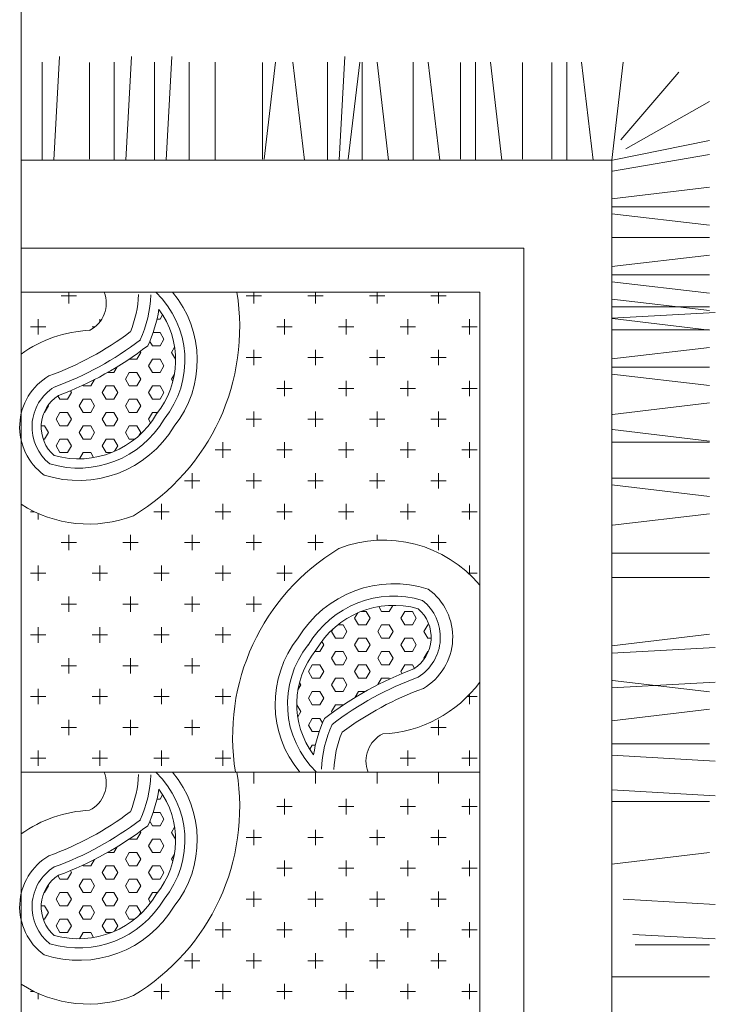
# Model space of a CAD drawing. Units: inches. Extents: x -638 to 186, y -762 to 59.
# Tile 26 of 31: x -65.1 to -52.81, y -94 to -76.62. Entities that reach past the tile are written whole.
import ezdxf

# ---------------------------------------------------------------- set-up
doc = ezdxf.new("R2010")
doc.units = ezdxf.units.IN
doc.layers.add('furn', color=8, linetype='Continuous', lineweight=13)

# ---------------------------------------------------------------- blocks, each defined once
blk = doc.blocks.new('BED-DOUBLE-WITH-NIGHTSTANDS')
for p, q in [((58.548, 11.244), (58.548, 59.951)), ((59.126, 31.914), (59.228, 33.743)), ((60.397, 31.914), (60.499, 33.743)), ((61.11, 31.914), (61.212, 33.743)), ((64.165, 31.914), (64.266, 33.743)), ((58.923, 31.914), (58.923, 33.642)), ((59.755, 31.928), (59.755, 33.639)), ((60.193, 31.914), (60.193, 33.642)), ((60.906, 31.914), (60.906, 33.642)), ((61.517, 31.914), (61.517, 33.642)), ((61.977, 31.914), (61.977, 33.642)), ((62.81, 31.928), (62.81, 33.639)), ((62.841, 31.928), (63.044, 33.642)), ((63.554, 31.914), (63.35, 33.642)), ((63.961, 31.914), (63.961, 33.642)), ((64.327, 31.928), (64.531, 33.642)), ((64.572, 31.914), (64.572, 33.642)), ((65.04, 31.914), (64.836, 33.642)), ((65.476, 31.914), (65.476, 33.642)), ((65.944, 31.914), (65.741, 33.642)), ((66.309, 31.928), (66.309, 33.639)), ((66.573, 31.914), (66.573, 33.642)), ((67.041, 31.914), (66.838, 33.642)), ((67.406, 31.928), (67.406, 33.639)), ((67.922, 31.928), (67.922, 33.639)), ((68.186, 31.914), (68.186, 33.642)), ((68.654, 31.914), (68.45, 33.642)), ((68.982, 31.914), (69.186, 33.642)), ((69.142, 32.273), (70.169, 33.468)), ((69.232, 32.112), (70.71, 32.951)), ((68.996, 31.914), (70.707, 32.257)), ((68.996, 31.721), (70.707, 32.011)), ((58.548, 31.914), (68.982, 31.914)), ((68.982, 31.914), (68.982, 1.829)), ((68.982, 31.232), (70.71, 31.436)), ((68.982, 30.966), (70.71, 30.762)), ((68.996, 31.086), (70.707, 31.086)), ((68.982, 30.547), (70.71, 30.547)), ((58.548, 30.359), (67.427, 30.359)), ((67.427, 30.359), (67.427, 3.384)), ((68.982, 30.033), (70.71, 30.237)), ((68.982, 29.767), (70.71, 29.563)), ((68.996, 29.887), (70.707, 29.887)), ((58.548, 29.582), (66.65, 29.582)), ((59.394, 29.379), (59.394, 29.582)), ((62.659, 29.379), (62.659, 29.582)), ((63.748, 29.379), (63.748, 29.582)), ((64.836, 29.379), (64.836, 29.582)), ((65.924, 29.379), (65.924, 29.582)), ((66.65, 29.582), (66.65, 4.161)), ((59.258, 29.515), (59.53, 29.515)), ((62.523, 29.515), (62.795, 29.515)), ((63.612, 29.515), (63.884, 29.515)), ((64.7, 29.515), (64.972, 29.515)), ((65.788, 29.515), (66.06, 29.515)), ((68.982, 29.46), (70.71, 29.256)), ((68.982, 29.324), (70.71, 29.324)), ((68.982, 29.121), (70.811, 29.223)), ((58.85, 28.835), (58.85, 29.107)), ((59.938, 29.054), (59.938, 29.107)), ((61.003, 29.104), (60.948, 29.104)), ((61.047, 29.18), (61.003, 29.104)), ((63.203, 28.835), (63.203, 29.107)), ((64.292, 28.835), (64.292, 29.107)), ((65.38, 28.835), (65.38, 29.107)), ((66.468, 28.835), (66.468, 29.107)), ((68.996, 29.116), (70.71, 28.912)), ((58.714, 28.971), (58.986, 28.971)), ((59.802, 28.971), (59.857, 28.971)), ((61.003, 28.869), (60.881, 28.869)), ((61.003, 28.869), (61.072, 28.751)), ((63.067, 28.971), (63.339, 28.971)), ((64.156, 28.971), (64.428, 28.971)), ((65.244, 28.971), (65.516, 28.971)), ((66.332, 28.971), (66.605, 28.971)), ((68.982, 28.917), (70.71, 28.917)), ((60.821, 28.713), (60.867, 28.633)), ((61.072, 28.751), (61.003, 28.633)), ((60.663, 28.515), (60.595, 28.397)), ((60.652, 28.534), (60.663, 28.515)), ((61.003, 28.633), (60.867, 28.633)), ((61.261, 28.608), (61.208, 28.515)), ((61.208, 28.515), (61.276, 28.397)), ((62.659, 28.291), (62.659, 28.563)), ((63.748, 28.291), (63.748, 28.563)), ((64.836, 28.291), (64.836, 28.563)), ((65.924, 28.291), (65.924, 28.563)), ((68.982, 28.403), (70.71, 28.606)), ((60.459, 28.399), (60.459, 28.397)), ((60.595, 28.397), (60.459, 28.397)), ((60.867, 28.397), (60.799, 28.28)), ((61.003, 28.397), (60.867, 28.397)), ((61.003, 28.397), (61.072, 28.28)), ((61.279, 28.397), (61.276, 28.397)), ((62.523, 28.427), (62.795, 28.427)), ((63.612, 28.427), (63.884, 28.427)), ((64.7, 28.427), (64.972, 28.427)), ((65.788, 28.427), (66.06, 28.427)), ((60.245, 28.262), (60.187, 28.162)), ((60.799, 28.28), (60.867, 28.162)), ((61.072, 28.28), (61.003, 28.162)), ((68.996, 28.256), (70.707, 28.256)), ((59.843, 28.037), (59.779, 27.926)), ((60.187, 28.162), (60.075, 28.162)), ((60.459, 28.162), (60.391, 28.044)), ((60.391, 28.044), (60.459, 27.926)), ((60.595, 28.162), (60.459, 28.162)), ((60.595, 28.162), (60.663, 28.044)), ((60.663, 28.044), (60.595, 27.926)), ((61.003, 28.162), (60.867, 28.162)), ((61.258, 28.131), (61.208, 28.044)), ((61.208, 28.044), (61.231, 28.004)), ((63.203, 27.747), (63.203, 28.019)), ((64.292, 27.747), (64.292, 28.019)), ((65.38, 27.747), (65.38, 28.019)), ((66.468, 27.747), (66.468, 28.019)), ((68.982, 28.136), (70.71, 27.933)), ((59.419, 27.842), (59.439, 27.808)), ((59.637, 27.937), (59.643, 27.926)), ((59.779, 27.926), (59.643, 27.926)), ((60.051, 27.926), (59.983, 27.808)), ((60.187, 27.926), (60.051, 27.926)), ((60.187, 27.926), (60.255, 27.808)), ((60.595, 27.926), (60.459, 27.926)), ((60.867, 27.926), (60.799, 27.808)), ((61.003, 27.926), (60.867, 27.926)), ((61.003, 27.926), (61.072, 27.808)), ((63.067, 27.883), (63.339, 27.883)), ((64.156, 27.883), (64.428, 27.883)), ((65.244, 27.883), (65.516, 27.883)), ((66.332, 27.883), (66.605, 27.883)), ((59.199, 27.753), (59.235, 27.69)), ((59.371, 27.69), (59.235, 27.69)), ((59.439, 27.808), (59.371, 27.69)), ((59.643, 27.69), (59.575, 27.573)), ((59.779, 27.69), (59.643, 27.69)), ((59.779, 27.69), (59.847, 27.573)), ((59.983, 27.808), (60.051, 27.69)), ((60.187, 27.69), (60.051, 27.69)), ((60.255, 27.808), (60.187, 27.69)), ((60.459, 27.69), (60.391, 27.573)), ((60.595, 27.69), (60.459, 27.69)), ((60.595, 27.69), (60.663, 27.573)), ((60.799, 27.808), (60.867, 27.69)), ((61.003, 27.69), (60.867, 27.69)), ((61.072, 27.808), (61.003, 27.69)), ((59.031, 27.573), (58.963, 27.455)), ((59.025, 27.583), (59.031, 27.573)), ((59.575, 27.573), (59.643, 27.455)), ((59.847, 27.573), (59.779, 27.455)), ((60.391, 27.573), (60.459, 27.455)), ((60.663, 27.573), (60.595, 27.455)), ((62.659, 27.203), (62.659, 27.475)), ((63.748, 27.203), (63.748, 27.475)), ((64.836, 27.203), (64.836, 27.475)), ((65.924, 27.203), (65.924, 27.475)), ((68.996, 27.424), (70.71, 27.627)), ((58.963, 27.455), (58.955, 27.455)), ((59.235, 27.455), (59.167, 27.337)), ((59.167, 27.337), (59.235, 27.219)), ((59.371, 27.455), (59.235, 27.455)), ((59.371, 27.455), (59.439, 27.337)), ((59.439, 27.337), (59.371, 27.219)), ((59.779, 27.455), (59.643, 27.455)), ((60.051, 27.455), (59.983, 27.337)), ((59.983, 27.337), (60.051, 27.219)), ((60.187, 27.455), (60.051, 27.455)), ((60.187, 27.455), (60.255, 27.337)), ((60.255, 27.337), (60.187, 27.219)), ((60.595, 27.455), (60.459, 27.455)), ((60.867, 27.455), (60.799, 27.337)), ((60.799, 27.337), (60.836, 27.274)), ((60.958, 27.455), (60.867, 27.455)), ((62.523, 27.339), (62.795, 27.339)), ((63.612, 27.339), (63.884, 27.339)), ((64.7, 27.339), (64.972, 27.339)), ((65.788, 27.339), (66.06, 27.339)), ((58.963, 27.219), (58.904, 27.219)), ((58.963, 27.219), (59.031, 27.101)), ((59.371, 27.219), (59.235, 27.219)), ((59.643, 27.219), (59.575, 27.101)), ((59.779, 27.219), (59.643, 27.219)), ((59.779, 27.219), (59.847, 27.101)), ((60.187, 27.219), (60.051, 27.219)), ((60.459, 27.219), (60.391, 27.101)), ((60.595, 27.219), (60.459, 27.219)), ((60.595, 27.219), (60.663, 27.101)), ((68.996, 27.156), (70.71, 26.953)), ((58.963, 26.984), (58.94, 26.984)), ((59.031, 27.101), (58.963, 26.984)), ((59.235, 26.984), (59.167, 26.866)), ((59.371, 26.984), (59.235, 26.984)), ((59.371, 26.984), (59.439, 26.866)), ((59.575, 27.101), (59.643, 26.984)), ((59.779, 26.984), (59.643, 26.984)), ((59.847, 27.101), (59.779, 26.984)), ((60.051, 26.984), (59.983, 26.866)), ((60.187, 26.984), (60.051, 26.984)), ((60.187, 26.984), (60.255, 26.866)), ((60.391, 27.101), (60.459, 26.984)), ((60.553, 26.984), (60.459, 26.984)), ((60.663, 27.101), (60.637, 27.055)), ((59.167, 26.866), (59.235, 26.748)), ((59.439, 26.866), (59.371, 26.748)), ((59.983, 26.866), (60.051, 26.748)), ((60.255, 26.866), (60.201, 26.772)), ((61.979, 26.795), (62.251, 26.795)), ((62.115, 26.659), (62.115, 26.931)), ((63.067, 26.795), (63.339, 26.795)), ((63.203, 26.659), (63.203, 26.931)), ((64.156, 26.795), (64.428, 26.795)), ((64.292, 26.659), (64.292, 26.931)), ((65.244, 26.795), (65.516, 26.795)), ((65.38, 26.659), (65.38, 26.931)), ((66.332, 26.795), (66.605, 26.795)), ((66.468, 26.659), (66.468, 26.931)), ((68.996, 26.933), (70.707, 26.933)), ((59.371, 26.748), (59.235, 26.748)), ((59.643, 26.748), (59.58, 26.638)), ((59.779, 26.748), (59.643, 26.748)), ((59.779, 26.748), (59.83, 26.661)), ((60.144, 26.748), (60.051, 26.748)), ((61.571, 26.114), (61.571, 26.386)), ((62.659, 26.114), (62.659, 26.386)), ((63.748, 26.114), (63.748, 26.386)), ((64.836, 26.114), (64.836, 26.386)), ((65.924, 26.114), (65.924, 26.386)), ((68.996, 26.297), (70.707, 26.297)), ((61.435, 26.25), (61.707, 26.25)), ((62.523, 26.25), (62.795, 26.25)), ((63.612, 26.25), (63.884, 26.25)), ((64.7, 26.25), (64.972, 26.25)), ((65.788, 26.25), (66.06, 26.25)), ((68.982, 26.177), (70.71, 25.974)), ((61.027, 25.57), (61.027, 25.842)), ((62.115, 25.57), (62.115, 25.842)), ((63.203, 25.57), (63.203, 25.842)), ((64.292, 25.57), (64.292, 25.842)), ((65.38, 25.57), (65.38, 25.842)), ((66.468, 25.57), (66.468, 25.842)), ((58.714, 25.706), (58.783, 25.706)), ((58.85, 25.57), (58.85, 25.675)), ((60.891, 25.706), (61.163, 25.706)), ((61.979, 25.706), (62.251, 25.706)), ((63.067, 25.706), (63.339, 25.706)), ((64.156, 25.706), (64.428, 25.706)), ((65.244, 25.706), (65.516, 25.706)), ((66.332, 25.706), (66.605, 25.706)), ((68.996, 25.465), (70.71, 25.668)), ((59.394, 25.026), (59.394, 25.298)), ((60.483, 25.026), (60.483, 25.298)), ((61.571, 25.026), (61.571, 25.298)), ((62.659, 25.026), (62.659, 25.298)), ((63.748, 25.026), (63.748, 25.298)), ((64.836, 25.2), (64.836, 25.298)), ((65.924, 25.026), (65.924, 25.298)), ((59.258, 25.162), (59.53, 25.162)), ((60.346, 25.162), (60.619, 25.162)), ((61.435, 25.162), (61.707, 25.162)), ((62.523, 25.162), (62.795, 25.162)), ((63.612, 25.162), (63.884, 25.162)), ((65.788, 25.162), (66.06, 25.162)), ((68.996, 24.973), (70.707, 24.973)), ((58.85, 24.482), (58.85, 24.754)), ((59.938, 24.482), (59.938, 24.754)), ((61.027, 24.482), (61.027, 24.754)), ((62.115, 24.482), (62.115, 24.754)), ((63.203, 24.482), (63.203, 24.754)), ((66.468, 24.601), (66.468, 24.754)), ((58.714, 24.618), (58.986, 24.618)), ((59.802, 24.618), (60.074, 24.618)), ((60.891, 24.618), (61.163, 24.618)), ((61.979, 24.618), (62.251, 24.618)), ((63.067, 24.618), (63.339, 24.618)), ((66.45, 24.618), (66.605, 24.618)), ((68.996, 24.543), (70.707, 24.543)), ((59.394, 23.938), (59.394, 24.21)), ((60.483, 23.938), (60.483, 24.21)), ((61.571, 23.938), (61.571, 24.21)), ((62.659, 23.938), (62.659, 24.21)), ((59.258, 24.074), (59.53, 24.074)), ((60.346, 24.074), (60.619, 24.074)), ((61.435, 24.074), (61.707, 24.074)), ((62.523, 24.074), (62.795, 24.074)), ((64.917, 23.942), (64.866, 24.03)), ((65.053, 23.942), (65.116, 24.052)), ((64.44, 23.825), (64.495, 23.919)), ((64.508, 23.707), (64.44, 23.825)), ((64.552, 23.942), (64.644, 23.942)), ((64.712, 23.825), (64.644, 23.942)), ((64.644, 23.707), (64.712, 23.825)), ((64.917, 23.942), (65.053, 23.942)), ((65.257, 23.825), (65.325, 23.942)), ((65.325, 23.707), (65.257, 23.825)), ((65.325, 23.942), (65.461, 23.942)), ((65.529, 23.825), (65.461, 23.942)), ((65.461, 23.707), (65.529, 23.825)), ((58.85, 23.393), (58.85, 23.666)), ((59.938, 23.393), (59.938, 23.666)), ((61.027, 23.393), (61.027, 23.666)), ((62.115, 23.393), (62.115, 23.666)), ((64.143, 23.707), (64.236, 23.707)), ((64.304, 23.589), (64.236, 23.707)), ((64.508, 23.707), (64.644, 23.707)), ((64.849, 23.589), (64.917, 23.707)), ((64.917, 23.707), (65.053, 23.707)), ((65.121, 23.589), (65.053, 23.707)), ((65.325, 23.707), (65.461, 23.707)), ((65.665, 23.589), (65.733, 23.707)), ((65.733, 23.707), (65.755, 23.707)), ((58.714, 23.53), (58.986, 23.53)), ((59.802, 23.53), (60.074, 23.53)), ((60.891, 23.53), (61.163, 23.53)), ((61.979, 23.53), (62.251, 23.53)), ((64.032, 23.589), (64.059, 23.635)), ((64.1, 23.471), (64.032, 23.589)), ((64.1, 23.471), (64.236, 23.471)), ((64.236, 23.471), (64.304, 23.589)), ((64.44, 23.353), (64.508, 23.471)), ((64.508, 23.471), (64.644, 23.471)), ((64.712, 23.353), (64.644, 23.471)), ((64.917, 23.471), (64.849, 23.589)), ((64.917, 23.471), (65.053, 23.471)), ((65.053, 23.471), (65.121, 23.589)), ((65.257, 23.353), (65.325, 23.471)), ((65.325, 23.471), (65.461, 23.471)), ((65.529, 23.353), (65.461, 23.471)), ((65.733, 23.471), (65.665, 23.589)), ((65.733, 23.471), (65.791, 23.471)), ((68.982, 23.339), (70.71, 23.542)), ((63.828, 23.235), (63.896, 23.353)), ((63.896, 23.353), (63.86, 23.416)), ((64.508, 23.235), (64.44, 23.353)), ((64.644, 23.235), (64.712, 23.353)), ((65.325, 23.235), (65.257, 23.353)), ((65.461, 23.235), (65.529, 23.353)), ((68.982, 23.207), (70.811, 23.309)), ((59.394, 22.849), (59.394, 23.121)), ((60.483, 22.849), (60.483, 23.121)), ((61.571, 22.849), (61.571, 23.121)), ((63.737, 23.235), (63.828, 23.235)), ((64.032, 23.118), (64.1, 23.235)), ((64.1, 23.235), (64.236, 23.235)), ((64.304, 23.118), (64.236, 23.235)), ((64.508, 23.235), (64.644, 23.235)), ((64.849, 23.118), (64.917, 23.235)), ((64.917, 23.235), (65.053, 23.235)), ((65.121, 23.118), (65.053, 23.235)), ((65.325, 23.235), (65.461, 23.235)), ((65.665, 23.118), (65.733, 23.235)), ((65.733, 23.235), (65.741, 23.235)), ((59.258, 22.985), (59.53, 22.985)), ((60.346, 22.985), (60.619, 22.985)), ((61.435, 22.985), (61.707, 22.985)), ((63.624, 22.882), (63.692, 23)), ((63.692, 23), (63.828, 23)), ((63.896, 22.882), (63.828, 23)), ((64.1, 23), (64.032, 23.118)), ((64.1, 23), (64.236, 23)), ((64.236, 23), (64.304, 23.118)), ((64.44, 22.882), (64.508, 23)), ((64.508, 23), (64.644, 23)), ((64.712, 22.882), (64.644, 23)), ((64.917, 23), (64.849, 23.118)), ((64.917, 23), (65.053, 23)), ((65.053, 23), (65.121, 23.118)), ((65.257, 22.882), (65.325, 23)), ((65.325, 23), (65.461, 23)), ((65.497, 22.937), (65.461, 23)), ((65.671, 23.107), (65.665, 23.118)), ((63.692, 22.764), (63.624, 22.882)), ((63.828, 22.764), (63.896, 22.882)), ((64.508, 22.764), (64.44, 22.882)), ((64.644, 22.764), (64.712, 22.882)), ((65.276, 22.848), (65.257, 22.882)), ((63.438, 22.559), (63.488, 22.646)), ((63.488, 22.646), (63.465, 22.686)), ((63.692, 22.764), (63.828, 22.764)), ((64.032, 22.646), (64.1, 22.764)), ((64.1, 22.529), (64.032, 22.646)), ((64.1, 22.764), (64.236, 22.764)), ((64.304, 22.646), (64.236, 22.764)), ((64.236, 22.529), (64.304, 22.646)), ((64.508, 22.764), (64.644, 22.764)), ((64.852, 22.653), (64.917, 22.764)), ((64.917, 22.764), (65.053, 22.764)), ((65.059, 22.753), (65.053, 22.764)), ((68.982, 22.596), (70.811, 22.698)), ((68.996, 22.728), (70.71, 22.524)), ((58.714, 22.441), (58.986, 22.441)), ((58.85, 22.305), (58.85, 22.577)), ((59.802, 22.441), (60.074, 22.441)), ((59.938, 22.305), (59.938, 22.577)), ((60.891, 22.441), (61.163, 22.441)), ((61.027, 22.305), (61.027, 22.577)), ((61.979, 22.441), (62.251, 22.441)), ((62.115, 22.305), (62.115, 22.577)), ((63.624, 22.411), (63.692, 22.529)), ((63.692, 22.529), (63.828, 22.529)), ((63.896, 22.411), (63.828, 22.529)), ((64.1, 22.529), (64.236, 22.529)), ((64.451, 22.428), (64.508, 22.529)), ((64.508, 22.529), (64.621, 22.529)), ((66.43, 22.441), (66.605, 22.441)), ((66.468, 22.305), (66.468, 22.481)), ((63.417, 22.293), (63.42, 22.293)), ((63.488, 22.175), (63.42, 22.293)), ((63.692, 22.293), (63.624, 22.411)), ((63.692, 22.293), (63.828, 22.293)), ((63.828, 22.293), (63.896, 22.411)), ((64.032, 22.175), (64.1, 22.293)), ((64.1, 22.293), (64.236, 22.293)), ((64.237, 22.292), (64.236, 22.293)), ((63.434, 22.082), (63.488, 22.175)), ((64.043, 22.156), (64.032, 22.175)), ((68.982, 22.015), (70.71, 22.219)), ((59.394, 21.761), (59.394, 22.033)), ((60.483, 21.761), (60.483, 22.033)), ((61.571, 21.761), (61.571, 22.033)), ((63.624, 21.939), (63.692, 22.057)), ((63.692, 21.822), (63.624, 21.939)), ((63.692, 22.057), (63.828, 22.057)), ((63.874, 21.977), (63.828, 22.057)), ((65.924, 21.761), (65.924, 22.033)), ((59.258, 21.897), (59.53, 21.897)), ((60.346, 21.897), (60.619, 21.897)), ((61.435, 21.897), (61.707, 21.897)), ((63.692, 21.822), (63.815, 21.822)), ((65.788, 21.897), (66.06, 21.897)), ((63.648, 21.51), (63.692, 21.586)), ((63.692, 21.586), (63.748, 21.586)), ((68.982, 21.608), (70.71, 21.608)), ((58.85, 21.217), (58.85, 21.489)), ((59.938, 21.217), (59.938, 21.489)), ((61.027, 21.217), (61.027, 21.489)), ((62.115, 21.217), (62.115, 21.489)), ((65.38, 21.217), (65.38, 21.489)), ((66.468, 21.217), (66.468, 21.489)), ((68.982, 21.404), (70.811, 21.302)), ((58.714, 21.353), (58.986, 21.353)), ((59.802, 21.353), (60.074, 21.353)), ((60.891, 21.353), (61.163, 21.353)), ((61.979, 21.353), (62.251, 21.353)), ((65.244, 21.353), (65.516, 21.353)), ((66.332, 21.353), (66.605, 21.353)), ((58.548, 21.108), (66.65, 21.108)), ((62.659, 20.906), (62.659, 21.108)), ((63.748, 20.906), (63.748, 21.108)), ((64.836, 20.906), (64.836, 21.108)), ((65.924, 20.906), (65.924, 21.108)), ((61.047, 20.707), (61.003, 20.631)), ((68.982, 20.793), (70.811, 20.691)), ((61.003, 20.631), (60.948, 20.631)), ((63.203, 20.362), (63.203, 20.634)), ((64.292, 20.362), (64.292, 20.634)), ((65.38, 20.362), (65.38, 20.634)), ((66.468, 20.362), (66.468, 20.634)), ((68.982, 20.59), (70.71, 20.59)), ((61.003, 20.395), (60.881, 20.395)), ((61.003, 20.395), (61.072, 20.277)), ((63.067, 20.498), (63.339, 20.498)), ((64.156, 20.498), (64.428, 20.498)), ((65.244, 20.498), (65.516, 20.498)), ((66.332, 20.498), (66.605, 20.498)), ((60.821, 20.239), (60.867, 20.159)), ((61.072, 20.277), (61.003, 20.159)), ((60.663, 20.042), (60.595, 19.924)), ((60.652, 20.061), (60.663, 20.042)), ((61.003, 20.159), (60.867, 20.159)), ((61.261, 20.135), (61.208, 20.042)), ((61.208, 20.042), (61.276, 19.924)), ((62.659, 19.817), (62.659, 20.09)), ((63.748, 19.817), (63.748, 20.09)), ((64.836, 19.817), (64.836, 20.09)), ((65.924, 19.817), (65.924, 20.09)), ((60.459, 19.925), (60.459, 19.924)), ((60.595, 19.924), (60.459, 19.924)), ((60.867, 19.924), (60.799, 19.806)), ((61.003, 19.924), (60.867, 19.924)), ((61.003, 19.924), (61.072, 19.806)), ((61.279, 19.924), (61.276, 19.924)), ((62.523, 19.954), (62.795, 19.954)), ((63.612, 19.954), (63.884, 19.954)), ((64.7, 19.954), (64.972, 19.954)), ((65.788, 19.954), (66.06, 19.954)), ((60.187, 19.688), (60.075, 19.688)), ((60.245, 19.788), (60.187, 19.688)), ((60.459, 19.688), (60.391, 19.57)), ((60.595, 19.688), (60.459, 19.688)), ((60.595, 19.688), (60.663, 19.57)), ((60.799, 19.806), (60.867, 19.688)), ((61.003, 19.688), (60.867, 19.688)), ((61.072, 19.806), (61.003, 19.688)), ((61.258, 19.657), (61.208, 19.57)), ((68.982, 19.485), (70.71, 19.689)), ((59.843, 19.564), (59.779, 19.453)), ((60.391, 19.57), (60.459, 19.453)), ((60.663, 19.57), (60.595, 19.453)), ((61.208, 19.57), (61.231, 19.53)), ((63.203, 19.273), (63.203, 19.545)), ((64.292, 19.273), (64.292, 19.545)), ((65.38, 19.273), (65.38, 19.545)), ((66.468, 19.273), (66.468, 19.545)), ((59.439, 19.335), (59.371, 19.217)), ((59.419, 19.369), (59.439, 19.335)), ((59.637, 19.464), (59.643, 19.453)), ((59.779, 19.453), (59.643, 19.453)), ((60.051, 19.453), (59.983, 19.335)), ((59.983, 19.335), (60.051, 19.217)), ((60.187, 19.453), (60.051, 19.453)), ((60.187, 19.453), (60.255, 19.335)), ((60.255, 19.335), (60.187, 19.217)), ((60.595, 19.453), (60.459, 19.453)), ((60.867, 19.453), (60.799, 19.335)), ((60.799, 19.335), (60.867, 19.217)), ((61.003, 19.453), (60.867, 19.453)), ((61.003, 19.453), (61.072, 19.335)), ((61.072, 19.335), (61.003, 19.217)), ((63.067, 19.409), (63.339, 19.409)), ((64.156, 19.409), (64.428, 19.409)), ((65.244, 19.409), (65.516, 19.409)), ((66.332, 19.409), (66.605, 19.409)), ((59.199, 19.28), (59.235, 19.217)), ((59.371, 19.217), (59.235, 19.217)), ((59.643, 19.217), (59.575, 19.099)), ((59.779, 19.217), (59.643, 19.217)), ((59.779, 19.217), (59.847, 19.099)), ((60.187, 19.217), (60.051, 19.217)), ((60.459, 19.217), (60.391, 19.099)), ((60.595, 19.217), (60.459, 19.217)), ((60.595, 19.217), (60.663, 19.099)), ((61.003, 19.217), (60.867, 19.217)), ((58.963, 18.981), (58.955, 18.981)), ((59.031, 19.099), (58.963, 18.981)), ((59.025, 19.109), (59.031, 19.099)), ((59.235, 18.981), (59.167, 18.863)), ((59.371, 18.981), (59.235, 18.981)), ((59.371, 18.981), (59.439, 18.863)), ((59.575, 19.099), (59.643, 18.981)), ((59.779, 18.981), (59.643, 18.981)), ((59.847, 19.099), (59.779, 18.981)), ((60.051, 18.981), (59.983, 18.863)), ((60.187, 18.981), (60.051, 18.981)), ((60.187, 18.981), (60.255, 18.863)), ((60.391, 19.099), (60.459, 18.981)), ((60.595, 18.981), (60.459, 18.981)), ((60.663, 19.099), (60.595, 18.981)), ((60.867, 18.981), (60.799, 18.863)), ((60.958, 18.981), (60.867, 18.981)), ((62.659, 18.729), (62.659, 19.001)), ((63.748, 18.729), (63.748, 19.001)), ((64.836, 18.729), (64.836, 19.001)), ((65.924, 18.729), (65.924, 19.001)), ((59.167, 18.863), (59.235, 18.746)), ((59.439, 18.863), (59.371, 18.746)), ((59.983, 18.863), (60.051, 18.746)), ((60.255, 18.863), (60.187, 18.746)), ((60.799, 18.863), (60.836, 18.801)), ((62.523, 18.865), (62.795, 18.865)), ((63.612, 18.865), (63.884, 18.865)), ((64.7, 18.865), (64.972, 18.865)), ((65.788, 18.865), (66.06, 18.865)), ((69.184, 18.863), (70.811, 18.772)), ((58.963, 18.746), (58.904, 18.746)), ((58.963, 18.746), (59.031, 18.628)), ((59.031, 18.628), (58.963, 18.51)), ((59.371, 18.746), (59.235, 18.746)), ((59.643, 18.746), (59.575, 18.628)), ((59.575, 18.628), (59.643, 18.51)), ((59.779, 18.746), (59.643, 18.746)), ((59.779, 18.746), (59.847, 18.628)), ((59.847, 18.628), (59.779, 18.51)), ((60.187, 18.746), (60.051, 18.746)), ((60.459, 18.746), (60.391, 18.628)), ((60.391, 18.628), (60.459, 18.51)), ((60.595, 18.746), (60.459, 18.746)), ((60.595, 18.746), (60.663, 18.628)), ((60.663, 18.628), (60.637, 18.582)), ((58.963, 18.51), (58.94, 18.51)), ((59.235, 18.51), (59.167, 18.392)), ((59.371, 18.51), (59.235, 18.51)), ((59.371, 18.51), (59.439, 18.392)), ((59.779, 18.51), (59.643, 18.51)), ((60.051, 18.51), (59.983, 18.392)), ((60.187, 18.51), (60.051, 18.51)), ((60.187, 18.51), (60.255, 18.392)), ((60.553, 18.51), (60.459, 18.51)), ((62.115, 18.185), (62.115, 18.457)), ((63.203, 18.185), (63.203, 18.457)), ((64.292, 18.185), (64.292, 18.457)), ((65.38, 18.185), (65.38, 18.457)), ((66.468, 18.185), (66.468, 18.457)), ((59.167, 18.392), (59.235, 18.274)), ((59.371, 18.274), (59.235, 18.274)), ((59.439, 18.392), (59.371, 18.274)), ((59.643, 18.274), (59.58, 18.165)), ((59.779, 18.274), (59.643, 18.274)), ((59.779, 18.274), (59.83, 18.187)), ((59.983, 18.392), (60.051, 18.274)), ((60.144, 18.274), (60.051, 18.274)), ((60.255, 18.392), (60.201, 18.298)), ((61.979, 18.321), (62.251, 18.321)), ((63.067, 18.321), (63.339, 18.321)), ((64.156, 18.321), (64.428, 18.321)), ((65.244, 18.321), (65.516, 18.321)), ((66.332, 18.321), (66.605, 18.321)), ((69.357, 18.243), (70.811, 18.162)), ((61.571, 17.641), (61.571, 17.913)), ((62.659, 17.641), (62.659, 17.913)), ((63.748, 17.641), (63.748, 17.913)), ((64.836, 17.641), (64.836, 17.913)), ((65.924, 17.641), (65.924, 17.913)), ((69.393, 18.06), (70.71, 18.06)), ((61.435, 17.777), (61.707, 17.777)), ((62.523, 17.777), (62.795, 17.777)), ((63.612, 17.777), (63.884, 17.777)), ((64.7, 17.777), (64.972, 17.777)), ((65.788, 17.777), (66.06, 17.777)), ((68.982, 17.492), (70.707, 17.492)), ((58.714, 17.233), (58.783, 17.233)), ((60.891, 17.233), (61.163, 17.233)), ((61.027, 17.097), (61.027, 17.369)), ((61.979, 17.233), (62.251, 17.233)), ((62.115, 17.097), (62.115, 17.369)), ((63.067, 17.233), (63.339, 17.233)), ((63.203, 17.097), (63.203, 17.369)), ((64.156, 17.233), (64.428, 17.233)), ((64.292, 17.097), (64.292, 17.369)), ((65.244, 17.233), (65.516, 17.233)), ((65.38, 17.097), (65.38, 17.369)), ((66.332, 17.233), (66.605, 17.233)), ((66.468, 17.097), (66.468, 17.369)), ((58.85, 17.097), (58.85, 17.202))]:
    blk.add_line(p, q)
for centre, radius, start, end in [((59.514, 29.388), 0.54, 297.0088, 21.0409), ((58.53, 28.957), 3.88, 301.1125, 9.2666), ((59.782, 28.381), 1.66, 321.1107, 46.3387), ((59.782, 28.381), 1.878, 321.5973, 39.7611), ((58.736, 29.604), 1.887, 337.4091, 358.0373), ((58.736, 29.604), 2.104, 335.7609, 358.0373), ((58.736, 29.604), 2.268, 334.7059, 351.7535), ((59.782, 28.381), 1.497, 320.6541, 36.833), ((59.856, 26.664), 2.246, 92.4675, 125.6302), ((57.143, 33.342), 5.571, 289.9219, 306.7677), ((57.143, 33.342), 5.789, 290.1318, 307.346), ((57.143, 33.342), 5.952, 290.2997, 307.7385), ((59.57, 27.2), 1.047, 120.344, 234.0192), ((59.57, 27.2), 0.829, 121.6232, 231.6957), ((59.57, 27.2), 0.666, 122.9498, 229.099), ((59.563, 28.229), 1.754, 253.2189, 329.4808), ((59.563, 28.229), 1.591, 254.3738, 329.9117), ((59.563, 28.229), 1.972, 252.055, 329.019), ((59.74, 27.689), 2.202, 237.1993, 291.1583), ((66.165, 21.733), 3.88, 121.1125, 189.2666), ((64.955, 23.002), 2.202, 39.6653, 111.1583), ((65.133, 22.461), 1.972, 72.055, 149.019), ((65.133, 22.461), 1.754, 73.2189, 149.4808), ((65.126, 23.49), 1.047, 300.344, 54.0192), ((65.133, 22.461), 1.591, 74.3738, 149.9117), ((65.126, 23.49), 0.666, 302.9498, 49.099), ((65.126, 23.49), 0.829, 301.6232, 51.6957), ((64.914, 22.31), 1.878, 141.5973, 219.7611), ((64.914, 22.31), 1.66, 141.1107, 226.3387), ((64.914, 22.31), 1.497, 140.6541, 216.833), ((67.553, 17.348), 5.952, 110.2997, 127.7385), ((67.553, 17.348), 5.789, 110.1318, 127.346), ((64.84, 24.027), 2.246, 272.4675, 323.7193), ((67.553, 17.348), 5.571, 109.9219, 126.7677), ((65.96, 21.087), 2.268, 154.7059, 171.7535), ((65.96, 21.087), 2.104, 155.7609, 178.0373), ((65.96, 21.087), 1.887, 157.4091, 178.0373), ((65.181, 21.302), 0.54, 117.0088, 201.0409), ((59.514, 20.915), 0.54, 297.0088, 21.0409), ((58.736, 21.13), 1.887, 337.4091, 358.0373), ((58.53, 20.484), 3.88, 301.1125, 9.2666), ((58.736, 21.13), 2.104, 335.7609, 358.0373), ((59.782, 19.907), 1.66, 321.1107, 46.3387), ((59.782, 19.907), 1.878, 321.5973, 39.7611), ((58.736, 21.13), 2.268, 334.7059, 351.7535), ((59.782, 19.907), 1.497, 320.6541, 36.833), ((59.856, 18.19), 2.246, 92.4675, 125.6302), ((57.143, 24.868), 5.571, 289.9219, 306.7677), ((57.143, 24.868), 5.789, 290.1318, 307.346), ((57.143, 24.868), 5.952, 290.2997, 307.7385), ((59.57, 18.727), 1.047, 120.344, 234.0192), ((59.57, 18.727), 0.829, 121.6232, 231.6957), ((59.57, 18.727), 0.666, 122.9498, 229.099), ((59.563, 19.756), 1.591, 254.3738, 329.9117), ((59.563, 19.756), 1.754, 253.2189, 329.4808), ((59.563, 19.756), 1.972, 252.055, 329.019), ((59.74, 19.215), 2.202, 237.1993, 291.1583)]:
    blk.add_arc(centre, radius, start, end)

msp = doc.modelspace()

# ---------------------------------------------------------------- block references
at = {"layer": 'furn'}
msp.add_blockref('BED-DOUBLE-WITH-NIGHTSTANDS', (-123.625, -111.013), dxfattribs=at)

doc.saveas('drawing.dxf')
